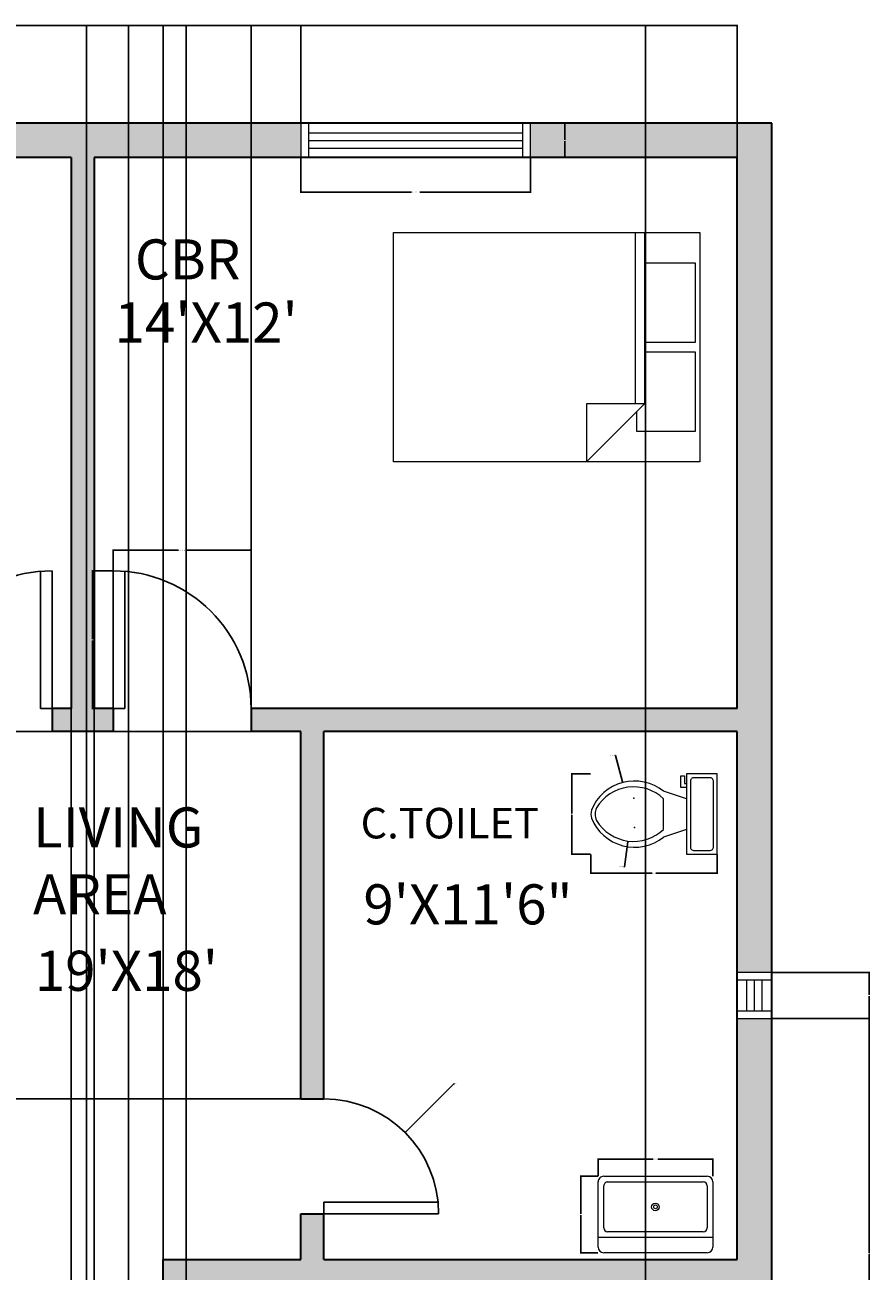
# Model space of a CAD drawing. Units: inches. Extents: x -82 to 330, y 553 to 1115.
# Tile 4 of 4: x 109 to 330, y 789 to 1115. Entities that reach past the tile are written whole.
import ezdxf

# ---------------------------------------------------------------- set-up
doc = ezdxf.new("R2010")
doc.units = ezdxf.units.IN
for name, color, linetype, lineweight in [('A-ANNO-DIMS', 2, 'Continuous', 18), ('A-AREA-IDEN', 7, 'Continuous', 25), ('A-DOOR', 3, 'Continuous', 25), ('A-FLOR-FIXT', 8, 'Continuous', 18), ('A-FURN', 8, 'Continuous', 18), ('A-GLAZ', 4, 'Continuous', 18), ('A-WALL', 7, 'Continuous', 35)]:
    doc.layers.add(name, color=color, linetype=linetype, lineweight=lineweight)
doc.layers.add('A-WALL-PATT', color=18, linetype='Continuous', lineweight=13, true_color=0x000000)
doc.styles.get("Standard").update_dxf_attribs({"font": 'arial.ttf'})
doc.dimstyles.get("Standard").update_dxf_attribs({"dimtxt": 0.18, "dimasz": 0.18, "dimexe": 0.18, "dimexo": 0.0625, "dimgap": 0.09, "dimtad": 0, "dimtih": 1, "dimtoh": 1, "dimdec": 4, "dimzin": 0, "dimdsep": 46, "dimtxsty": 'Standard', "dimcen": 0.09, "dimadec": 0, "dimazin": 0, "dimtfac": 1, "dimtdec": 4, "dimtofl": 0, "dimtmove": 0, "dimatfit": 3, "dimfxl": 1, "dimtolj": 1, "dimtzin": 0, "dimarcsym": 0})

# ---------------------------------------------------------------- blocks, each defined once
blk = doc.blocks.new('Sink-single - 30 in top')
blk.add_line((-15, -3.999996), (15, -3.999996))
for points in [[(-13.5, 0), (13.5, 0)], [(-15, -18.499996), (-15, -1.5)], [(15, -1.5), (15, -18.499996)], [(-13.5, -17.499996), (-13.5, -6.499996)], [(-12.5, -5.499996), (12.5, -5.499996)], [(13.5, -6.499996), (13.5, -17.499996)], [(12.5, -18.499996), (-12.5, -18.499996)], [(13.5, -19.999996), (-13.5, -19.999996)]]:
    blk.add_lwpolyline(points)
for radius in [1, 0.5]:
    blk.add_circle((0, -11.999996), radius)
for centre, radius, start, end in [((-13.5, -1.5), 1.5, 90, 180), ((13.5, -1.5), 1.5, 0, 90), ((-12.5, -6.499996), 1, 90, 180), ((12.5, -6.499996), 1, 0, 90), ((-13.5, -18.499996), 1.5, 180, 270), ((-12.5, -17.499996), 1, 180, 270), ((12.5, -17.499996), 1, 270, 0), ((13.5, -18.499996), 1.5, 270, 0)]:
    blk.add_arc(centre, radius, start, end)
blk = doc.blocks.new('Bed - Queen')
for p, q in [((0, -80.00003), (0, 0)), ((0, 0), (59.99999, 0)), ((59.99999, 0), (59.99999, -80.00003)), ((7.99999, -1.2), (28.79998, -1.2)), ((7.99999, -14.4), (7.99999, -1.2)), ((28.79998, -1.2), (28.79998, -14.4)), ((31.19999, -1.2), (51.99999, -1.2)), ((31.19999, -14.4), (31.19999, -1.2)), ((51.99999, -1.2), (51.99999, -16.4)), ((0, -14.4), (44.8, -14.4)), ((59.99999, -29.6), (44.8, -14.4)), ((44.8, -14.4), (44.8, -29.6)), ((44.8, -16.8), (0, -16.8)), ((51.99999, -16.4), (46.79936, -16.4)), ((44.8, -29.6), (59.99999, -29.6)), ((59.99999, -80.00003), (0, -80.00003))]:
    blk.add_line(p, q)
blk = doc.blocks.new('Toilet - top')
for p, q in [((9.5, -6), (9.5, -2)), ((-10, -8.5), (-8, -8.5)), ((-10, -9.5), (-10, -8.5)), ((-7, -9.5), (-10, -9.5)), ((-8, -8.5), (-8, -8)), ((-7, -8), (-7, -9.5)), ((-4, -8), (-6, -14)), ((4, -8), (6, -14)), ((4, -14), (-4, -14))]:
    blk.add_line(p, q)
blk.add_lwpolyline([(10.5, -8), (10.5, 0), (-10.5, 0), (-10.5, -8)], close=True)
for points in [[(-9.5, -2), (-9.5, -6)], [(8.5, -1), (-8.5, -1)], [(-8.5, -7), (8.5, -7)]]:
    blk.add_lwpolyline(points)
for centre, radius, start, end in [((-8.62, -1.88), 0.884, 81.8699, 188.1301), ((8.62, -1.88), 0.884, 351.8699, 98.1301), ((-8.62, -6.12), 0.884, 171.8699, 278.1301), ((8.62, -6.12), 0.884, 261.8699, 8.1301), ((3.52, -21.58), 12.17, 141.4691, 247.9714), ((4.2, -21.82), 11.33, 136.3677, 238.9468), ((-3.52, -21.58), 12.17, 292.0284, 38.5307), ((-4.2, -21.82), 11.33, 301.053, 43.6321), ((0, -27.88), 4, 245.7318, 294.2682), ((0, -29), 4, 254.8605, 285.1395)]:
    blk.add_arc(centre, radius, start, end)
blk = doc.blocks.new('WIN-60IN')
for p, q in [((60, 9), (0, 9)), ((0, 9), (0, 0)), ((2, 9), (2, 0)), ((58, 0), (58, 9)), ((60, 0), (60, 9)), ((2, 6.5), (58, 6.5)), ((2, 4.5), (58, 4.5)), ((0, 0), (60, 0)), ((2, 2.5), (58, 2.5))]:
    blk.add_line(p, q)
blk = doc.blocks.new('DOOR-SWING-36IN')
for p, q in [((0, 36), (0, 0)), ((3, 36), (3, 0)), ((0, 0), (3, 0))]:
    blk.add_line(p, q)
blk.add_arc((0, 0), 36, 0, 90)
blk = doc.blocks.new('*D11')
at = {"layer": 'A-ANNO-DIMS', "color": 0, "lineweight": -2, "transparency": 16777216}
for p, q in [((180.99, 1080.05), (180.99, 1070.93)), ((240.99, 1080.05), (240.99, 1070.93)), ((181.17, 1071.11), (209.87, 1071.11)), ((240.81, 1071.11), (212.11, 1071.11))]:
    blk.add_line(p, q, dxfattribs=at)
at = {"layer": 'A-ANNO-DIMS', "color": 0, "transparency": 16777216}
for points in [[(181.17, 1071.14), (181.17, 1071.08), (180.99, 1071.11)], [(240.81, 1071.14), (240.81, 1071.08), (240.99, 1071.11)]]:
    blk.add_solid(points, dxfattribs=at)
at = {"layer": 'Defpoints', "color": 0, "transparency": 16777216}
for p in [(180.99, 1080.11), (240.99, 1080.11), (240.99, 1071.11)]:
    blk.add_point(p, dxfattribs=at)
at = {"layer": 'A-ANNO-DIMS', "color": 0, "transparency": 16777216, "insert": (210.99, 1071.11), "char_height": 0.18, "attachment_point": 5}
blk.add_mtext('\\A1;WINDOW 60 TYP.', dxfattribs=at)
blk = doc.blocks.new('*D12')
at = {"layer": 'A-ANNO-DIMS', "color": 0, "lineweight": -2, "transparency": 16777216}
for p, q in [((241.05, 1089.11), (250.17, 1089.11)), ((249.99, 1088.93), (249.99, 1084.79)), ((249.99, 1080.29), (249.99, 1084.43)), ((241.05, 1080.11), (250.17, 1080.11))]:
    blk.add_line(p, q, dxfattribs=at)
at = {"layer": 'A-ANNO-DIMS', "color": 0, "transparency": 16777216}
for points in [[(249.96, 1088.93), (250.02, 1088.93), (249.99, 1089.11)], [(249.96, 1080.29), (250.02, 1080.29), (249.99, 1080.11)]]:
    blk.add_solid(points, dxfattribs=at)
at = {"layer": 'Defpoints', "color": 0, "transparency": 16777216}
for p in [(240.99, 1089.11), (249.99, 1089.11), (240.99, 1080.11)]:
    blk.add_point(p, dxfattribs=at)
at = {"layer": 'A-ANNO-DIMS', "color": 0, "transparency": 16777216, "insert": (249.99, 1084.61), "char_height": 0.18, "attachment_point": 5}
blk.add_mtext('\\A1;9 TYP.', dxfattribs=at)
blk = doc.blocks.new('*D13')
at = {"layer": 'A-ANNO-DIMS', "color": 0, "lineweight": -2, "transparency": 16777216}
for p, q in [((131.99, 972.17), (131.99, 977.69)), ((132.17, 977.51), (149.05, 977.51)), ((167.81, 977.51), (150.92, 977.51)), ((167.99, 972.17), (167.99, 977.69))]:
    blk.add_line(p, q, dxfattribs=at)
at = {"layer": 'A-ANNO-DIMS', "color": 0, "transparency": 16777216}
for points in [[(132.17, 977.54), (132.17, 977.48), (131.99, 977.51)], [(167.81, 977.54), (167.81, 977.48), (167.99, 977.51)]]:
    blk.add_solid(points, dxfattribs=at)
at = {"layer": 'Defpoints', "color": 0, "transparency": 16777216}
for p in [(167.99, 977.51), (131.99, 972.11), (167.99, 972.11)]:
    blk.add_point(p, dxfattribs=at)
at = {"layer": 'A-ANNO-DIMS', "color": 0, "transparency": 16777216, "insert": (149.99, 977.51), "char_height": 0.18, "attachment_point": 5}
blk.add_mtext('\\A1;DOOR 36 TYP.', dxfattribs=at)
blk = doc.blocks.new('*D14')
at = {"layer": 'A-ANNO-DIMS', "color": 0, "lineweight": -2, "transparency": 16777216}
for p, q in [((131.93, 972.11), (126.41, 972.11)), ((126.59, 971.93), (126.59, 954.29)), ((126.59, 936.29), (126.59, 953.93)), ((131.93, 936.11), (126.41, 936.11))]:
    blk.add_line(p, q, dxfattribs=at)
at = {"layer": 'A-ANNO-DIMS', "color": 0, "transparency": 16777216}
for points in [[(126.56, 971.93), (126.62, 971.93), (126.59, 972.11)], [(126.56, 936.29), (126.62, 936.29), (126.59, 936.11)]]:
    blk.add_solid(points, dxfattribs=at)
at = {"layer": 'Defpoints', "color": 0, "transparency": 16777216}
for p in [(126.59, 972.11), (131.99, 972.11), (131.99, 936.11)]:
    blk.add_point(p, dxfattribs=at)
at = {"layer": 'A-ANNO-DIMS', "color": 0, "transparency": 16777216, "insert": (126.59, 954.11), "char_height": 0.18, "attachment_point": 5}
blk.add_mtext('\\A1;36 TYP.', dxfattribs=at)
blk = doc.blocks.new('*D23')
at = {"layer": 'A-ANNO-DIMS', "color": 0, "lineweight": -2, "transparency": 16777216}
for p, q in [((258.63, 813.95), (258.63, 818.57)), ((258.81, 818.39), (273, 818.39)), ((288.45, 818.39), (274.26, 818.39)), ((288.63, 813.95), (288.63, 818.57))]:
    blk.add_line(p, q, dxfattribs=at)
at = {"layer": 'A-ANNO-DIMS', "color": 0, "transparency": 16777216}
for points in [[(258.81, 818.42), (258.81, 818.36), (258.63, 818.39)], [(288.45, 818.42), (288.45, 818.36), (288.63, 818.39)]]:
    blk.add_solid(points, dxfattribs=at)
at = {"layer": 'Defpoints', "color": 0, "transparency": 16777216}
for p in [(258.63, 818.39), (258.63, 813.89), (288.63, 813.89)]:
    blk.add_point(p, dxfattribs=at)
at = {"layer": 'A-ANNO-DIMS', "color": 0, "transparency": 16777216, "insert": (273.63, 818.39), "char_height": 0.18, "attachment_point": 5}
blk.add_mtext('\\A1;BASIN 30', dxfattribs=at)
blk = doc.blocks.new('*D24')
at = {"layer": 'A-ANNO-DIMS', "color": 0, "lineweight": -2, "transparency": 16777216}
for p, q in [((258.57, 813.89), (253.95, 813.89)), ((254.13, 813.71), (254.13, 804.07)), ((254.13, 794.07), (254.13, 803.71)), ((258.57, 793.89), (253.95, 793.89))]:
    blk.add_line(p, q, dxfattribs=at)
at = {"layer": 'A-ANNO-DIMS', "color": 0, "transparency": 16777216}
for points in [[(254.1, 813.71), (254.16, 813.71), (254.13, 813.89)], [(254.1, 794.07), (254.16, 794.07), (254.13, 793.89)]]:
    blk.add_solid(points, dxfattribs=at)
at = {"layer": 'Defpoints', "color": 0, "transparency": 16777216}
for p in [(258.63, 813.89), (254.13, 793.89), (258.63, 793.89)]:
    blk.add_point(p, dxfattribs=at)
at = {"layer": 'A-ANNO-DIMS', "color": 0, "transparency": 16777216, "insert": (254.13, 803.89), "char_height": 0.18, "attachment_point": 5}
blk.add_mtext('\\A1;20', dxfattribs=at)
blk = doc.blocks.new('*D29')
at = {"layer": 'A-ANNO-DIMS', "color": 0, "lineweight": -2, "transparency": 16777216}
for p, q in [((256.71, 897.97), (256.71, 892.9)), ((289.76, 897.97), (289.76, 892.9)), ((256.89, 893.08), (272.77, 893.08)), ((289.58, 893.08), (273.7, 893.08))]:
    blk.add_line(p, q, dxfattribs=at)
at = {"layer": 'A-ANNO-DIMS', "color": 0, "transparency": 16777216}
for points in [[(256.89, 893.11), (256.89, 893.05), (256.71, 893.08)], [(289.58, 893.11), (289.58, 893.05), (289.76, 893.08)]]:
    blk.add_solid(points, dxfattribs=at)
at = {"layer": 'Defpoints', "color": 0, "transparency": 16777216}
for p in [(256.71, 898.03), (289.76, 898.03), (289.76, 893.08)]:
    blk.add_point(p, dxfattribs=at)
at = {"layer": 'A-ANNO-DIMS', "color": 0, "transparency": 16777216, "insert": (273.23, 893.08), "char_height": 0.18, "attachment_point": 5}
blk.add_mtext('\\A1;WC 33', dxfattribs=at)
blk = doc.blocks.new('*D30')
at = {"layer": 'A-ANNO-DIMS', "color": 0, "lineweight": -2, "transparency": 16777216}
for p, q in [((256.65, 919.03), (251.57, 919.03)), ((251.75, 918.85), (251.75, 908.72)), ((251.75, 898.21), (251.75, 908.35)), ((256.65, 898.03), (251.57, 898.03))]:
    blk.add_line(p, q, dxfattribs=at)
at = {"layer": 'A-ANNO-DIMS', "color": 0, "transparency": 16777216}
for points in [[(251.72, 918.85), (251.78, 918.85), (251.75, 919.03)], [(251.72, 898.21), (251.78, 898.21), (251.75, 898.03)]]:
    blk.add_solid(points, dxfattribs=at)
at = {"layer": 'Defpoints', "color": 0, "transparency": 16777216}
for p in [(256.71, 919.03), (251.75, 898.03), (256.71, 898.03)]:
    blk.add_point(p, dxfattribs=at)
at = {"layer": 'A-ANNO-DIMS', "color": 0, "transparency": 16777216, "insert": (251.75, 908.53), "char_height": 0.18, "attachment_point": 5}
blk.add_mtext('\\A1;21', dxfattribs=at)
blk = doc.blocks.new('*D34')
at = {"layer": 'A-ANNO-DIMS', "color": 0, "lineweight": -2, "transparency": 16777216}
for p, q in [((66.99, 1089.17), (66.99, 1114.79)), ((67.17, 1114.61), (123.71, 1114.61)), ((180.81, 1114.61), (124.27, 1114.61)), ((180.99, 1089.17), (180.99, 1114.79))]:
    blk.add_line(p, q, dxfattribs=at)
at = {"layer": 'A-ANNO-DIMS', "color": 0, "transparency": 16777216}
for points in [[(67.17, 1114.64), (67.17, 1114.58), (66.99, 1114.61)], [(180.81, 1114.64), (180.81, 1114.58), (180.99, 1114.61)]]:
    blk.add_solid(points, dxfattribs=at)
at = {"layer": 'Defpoints', "color": 0, "transparency": 16777216}
for p in [(180.99, 1114.61), (66.99, 1089.11), (180.99, 1089.11)]:
    blk.add_point(p, dxfattribs=at)
at = {"layer": 'A-ANNO-DIMS', "color": 0, "transparency": 16777216, "insert": (123.99, 1114.61), "char_height": 0.18, "attachment_point": 5}
blk.add_mtext('\\A1;114', dxfattribs=at)
blk = doc.blocks.new('*D35')
at = {"layer": 'A-ANNO-DIMS', "color": 0, "lineweight": -2, "transparency": 16777216}
for p, q in [((84.99, 627.17), (84.99, 1114.79)), ((85.17, 1114.61), (110.29, 1114.61)), ((135.81, 1114.61), (110.69, 1114.61)), ((135.99, 618.17), (135.99, 1114.79))]:
    blk.add_line(p, q, dxfattribs=at)
at = {"layer": 'A-ANNO-DIMS', "color": 0, "transparency": 16777216}
for points in [[(85.17, 1114.64), (85.17, 1114.58), (84.99, 1114.61)], [(135.81, 1114.64), (135.81, 1114.58), (135.99, 1114.61)]]:
    blk.add_solid(points, dxfattribs=at)
at = {"layer": 'Defpoints', "color": 0, "transparency": 16777216}
for p in [(135.99, 1114.61), (84.99, 627.11), (135.99, 618.11)]:
    blk.add_point(p, dxfattribs=at)
at = {"layer": 'A-ANNO-DIMS', "color": 0, "transparency": 16777216, "insert": (110.49, 1114.61), "char_height": 0.18, "attachment_point": 5}
blk.add_mtext('\\A1;51', dxfattribs=at)
blk = doc.blocks.new('*D39')
at = {"layer": 'A-ANNO-DIMS', "color": 0, "lineweight": -2, "transparency": 16777216}
for p, q in [((304.05, 855.11), (329.67, 855.11)), ((329.49, 854.93), (329.49, 793.79)), ((329.49, 732.29), (329.49, 793.43)), ((304.05, 732.11), (329.67, 732.11))]:
    blk.add_line(p, q, dxfattribs=at)
at = {"layer": 'A-ANNO-DIMS', "color": 0, "transparency": 16777216}
for points in [[(329.46, 854.93), (329.52, 854.93), (329.49, 855.11)], [(329.46, 732.29), (329.52, 732.29), (329.49, 732.11)]]:
    blk.add_solid(points, dxfattribs=at)
at = {"layer": 'Defpoints', "color": 0, "transparency": 16777216}
for p in [(303.99, 855.11), (329.49, 855.11), (303.99, 732.11)]:
    blk.add_point(p, dxfattribs=at)
at = {"layer": 'A-ANNO-DIMS', "color": 0, "transparency": 16777216, "insert": (329.49, 793.61), "char_height": 0.18, "attachment_point": 5}
blk.add_mtext('\\A1;123', dxfattribs=at)
blk = doc.blocks.new('*D40')
at = {"layer": 'A-ANNO-DIMS', "color": 0, "lineweight": -2, "transparency": 16777216}
for p, q in [((304.05, 867.11), (329.67, 867.11)), ((329.49, 866.93), (329.49, 861.29)), ((329.49, 855.29), (329.49, 860.93)), ((304.05, 855.11), (329.67, 855.11))]:
    blk.add_line(p, q, dxfattribs=at)
at = {"layer": 'A-ANNO-DIMS', "color": 0, "transparency": 16777216}
for points in [[(329.46, 866.93), (329.52, 866.93), (329.49, 867.11)], [(329.46, 855.29), (329.52, 855.29), (329.49, 855.11)]]:
    blk.add_solid(points, dxfattribs=at)
at = {"layer": 'Defpoints', "color": 0, "transparency": 16777216}
for p in [(303.99, 867.11), (329.49, 867.11), (303.99, 855.11)]:
    blk.add_point(p, dxfattribs=at)
at = {"layer": 'A-ANNO-DIMS', "color": 0, "transparency": 16777216, "insert": (329.49, 861.11), "char_height": 0.18, "attachment_point": 5}
blk.add_mtext('\\A1;12', dxfattribs=at)
blk = doc.blocks.new('*D41')
at = {"layer": 'A-ANNO-DIMS', "color": 0, "lineweight": -2, "transparency": 16777216}
for p, q in [((124.99, 714.17), (124.99, 1114.79)), ((125.17, 1114.61), (134.77, 1114.61)), ((144.81, 1114.61), (135.21, 1114.61)), ((144.99, 714.17), (144.99, 1114.79))]:
    blk.add_line(p, q, dxfattribs=at)
at = {"layer": 'A-ANNO-DIMS', "color": 0, "transparency": 16777216}
for points in [[(125.17, 1114.64), (125.17, 1114.58), (124.99, 1114.61)], [(144.81, 1114.64), (144.81, 1114.58), (144.99, 1114.61)]]:
    blk.add_solid(points, dxfattribs=at)
at = {"layer": 'Defpoints', "color": 0, "transparency": 16777216}
for p in [(144.99, 1114.61), (124.99, 714.11), (144.99, 714.11)]:
    blk.add_point(p, dxfattribs=at)
at = {"layer": 'A-ANNO-DIMS', "color": 0, "transparency": 16777216, "insert": (134.99, 1114.61), "char_height": 0.18, "attachment_point": 5}
blk.add_mtext('\\A1;20', dxfattribs=at)
blk = doc.blocks.new('*D43')
at = {"layer": 'A-ANNO-DIMS', "color": 0, "lineweight": -2, "transparency": 16777216}
for p, q in [((120.99, 1080.05), (120.99, 553.43)), ((126.99, 1080.05), (126.99, 553.43)), ((121.17, 553.61), (123.84, 553.61)), ((126.81, 553.61), (124.14, 553.61))]:
    blk.add_line(p, q, dxfattribs=at)
at = {"layer": 'A-ANNO-DIMS', "color": 0, "transparency": 16777216}
for points in [[(121.17, 553.64), (121.17, 553.58), (120.99, 553.61)], [(126.81, 553.64), (126.81, 553.58), (126.99, 553.61)]]:
    blk.add_solid(points, dxfattribs=at)
at = {"layer": 'Defpoints', "color": 0, "transparency": 16777216}
for p in [(120.99, 1080.11), (126.99, 1080.11), (126.99, 553.61)]:
    blk.add_point(p, dxfattribs=at)
at = {"layer": 'A-ANNO-DIMS', "color": 0, "transparency": 16777216, "insert": (123.99, 553.61), "char_height": 0.18, "attachment_point": 5}
blk.add_mtext('\\A1;6', dxfattribs=at)
blk = doc.blocks.new('*D45')
at = {"layer": 'A-ANNO-DIMS', "color": 0, "lineweight": -2, "transparency": 16777216}
for p, q in [((180.93, 930.11), (-81.69, 930.11)), ((-81.51, 929.93), (-81.51, 882.29)), ((-81.51, 834.29), (-81.51, 881.93)), ((180.93, 834.11), (-81.69, 834.11))]:
    blk.add_line(p, q, dxfattribs=at)
at = {"layer": 'A-ANNO-DIMS', "color": 0, "transparency": 16777216}
for points in [[(-81.54, 929.93), (-81.48, 929.93), (-81.51, 930.11)], [(-81.54, 834.29), (-81.48, 834.29), (-81.51, 834.11)]]:
    blk.add_solid(points, dxfattribs=at)
at = {"layer": 'Defpoints', "color": 0, "transparency": 16777216}
for p in [(180.99, 930.11), (-81.51, 834.11), (180.99, 834.11)]:
    blk.add_point(p, dxfattribs=at)
at = {"layer": 'A-ANNO-DIMS', "color": 0, "transparency": 16777216, "insert": (-81.51, 882.11), "char_height": 0.18, "attachment_point": 5}
blk.add_mtext('\\A1;96', dxfattribs=at)
blk = doc.blocks.new('*D47')
at = {"layer": 'A-ANNO-DIMS', "color": 0, "lineweight": -2, "transparency": 16777216}
for p, q in [((167.99, 936.17), (167.99, 1114.79)), ((168.17, 1114.61), (231.21, 1114.61)), ((294.81, 1114.61), (231.77, 1114.61)), ((294.99, 936.17), (294.99, 1114.79))]:
    blk.add_line(p, q, dxfattribs=at)
at = {"layer": 'A-ANNO-DIMS', "color": 0, "transparency": 16777216}
for points in [[(168.17, 1114.64), (168.17, 1114.58), (167.99, 1114.61)], [(294.81, 1114.64), (294.81, 1114.58), (294.99, 1114.61)]]:
    blk.add_solid(points, dxfattribs=at)
at = {"layer": 'Defpoints', "color": 0, "transparency": 16777216}
for p in [(294.99, 1114.61), (167.99, 936.11), (294.99, 936.11)]:
    blk.add_point(p, dxfattribs=at)
at = {"layer": 'A-ANNO-DIMS', "color": 0, "transparency": 16777216, "insert": (231.49, 1114.61), "char_height": 0.18, "attachment_point": 5}
blk.add_mtext('\\A1;127', dxfattribs=at)
blk = doc.blocks.new('*D48')
at = {"layer": 'A-ANNO-DIMS', "color": 0, "lineweight": -2, "transparency": 16777216}
for p, q in [((-50.01, 609.17), (-50.01, 1114.79)), ((-49.83, 1114.61), (42.71, 1114.61)), ((135.81, 1114.61), (43.27, 1114.61)), ((135.99, 618.17), (135.99, 1114.79))]:
    blk.add_line(p, q, dxfattribs=at)
at = {"layer": 'A-ANNO-DIMS', "color": 0, "transparency": 16777216}
for points in [[(-49.83, 1114.64), (-49.83, 1114.58), (-50.01, 1114.61)], [(135.81, 1114.64), (135.81, 1114.58), (135.99, 1114.61)]]:
    blk.add_solid(points, dxfattribs=at)
at = {"layer": 'Defpoints', "color": 0, "transparency": 16777216}
for p in [(135.99, 1114.61), (135.99, 618.11), (-50.01, 609.11)]:
    blk.add_point(p, dxfattribs=at)
at = {"layer": 'A-ANNO-DIMS', "color": 0, "transparency": 16777216, "insert": (42.99, 1114.61), "char_height": 0.18, "attachment_point": 5}
blk.add_mtext('\\A1;186', dxfattribs=at)
blk = doc.blocks.new('*D49')
at = {"layer": 'A-ANNO-DIMS', "color": 0, "lineweight": -2, "transparency": 16777216}
for p, q in [((150.99, 642.17), (150.99, 1114.79)), ((151.17, 1114.61), (210.71, 1114.61)), ((270.81, 1114.61), (211.27, 1114.61)), ((270.99, 642.17), (270.99, 1114.79))]:
    blk.add_line(p, q, dxfattribs=at)
at = {"layer": 'A-ANNO-DIMS', "color": 0, "transparency": 16777216}
for points in [[(151.17, 1114.64), (151.17, 1114.58), (150.99, 1114.61)], [(270.81, 1114.64), (270.81, 1114.58), (270.99, 1114.61)]]:
    blk.add_solid(points, dxfattribs=at)
at = {"layer": 'Defpoints', "color": 0, "transparency": 16777216}
for p in [(270.99, 1114.61), (150.99, 642.11), (270.99, 642.11)]:
    blk.add_point(p, dxfattribs=at)
at = {"layer": 'A-ANNO-DIMS', "color": 0, "transparency": 16777216, "insert": (210.99, 1114.61), "char_height": 0.18, "attachment_point": 5}
blk.add_mtext('\\A1;120', dxfattribs=at)
blk = doc.blocks.new('*D51')
at = {"layer": 'A-ANNO-DIMS', "color": 0, "lineweight": -2, "transparency": 16777216}
for p, q in [((220.93, 838.05), (208.33, 825.45)), ((221.11, 838.05), (220.93, 838.05)), ((186.9, 804.11), (187.08, 804.11)), ((186.99, 804.02), (186.99, 804.2))]:
    blk.add_line(p, q, dxfattribs=at)
at = {"layer": 'A-ANNO-DIMS', "color": 0, "transparency": 16777216}
blk.add_solid([(208.31, 825.47), (208.35, 825.43), (208.2, 825.32)], dxfattribs=at)
at = {"layer": 'Defpoints', "color": 0, "transparency": 16777216}
for p in [(208.2, 825.32), (186.99, 804.11)]:
    blk.add_point(p, dxfattribs=at)
at = {"layer": 'A-ANNO-DIMS', "color": 0, "transparency": 16777216, "insert": (221.41, 838.05), "char_height": 0.18, "attachment_point": 5}
blk.add_mtext('\\A1;R30', dxfattribs=at)
blk = doc.blocks.new('*D52')
at = {"layer": 'A-ANNO-DIMS', "color": 0, "lineweight": -2, "transparency": 16777216}
for p, q in [((263.05, 923.85), (263.23, 923.85)), ((263.23, 923.85), (265.04, 916.96)), ((268.09, 905.02), (268.27, 905.02)), ((268.18, 904.93), (268.18, 905.11))]:
    blk.add_line(p, q, dxfattribs=at)
at = {"layer": 'A-ANNO-DIMS', "color": 0, "transparency": 16777216}
blk.add_solid([(265.07, 916.97), (265.01, 916.95), (265.08, 916.78)], dxfattribs=at)
at = {"layer": 'Defpoints', "color": 0, "transparency": 16777216}
for p in [(265.08, 916.78), (268.18, 905.02)]:
    blk.add_point(p, dxfattribs=at)
at = {"layer": 'A-ANNO-DIMS', "color": 0, "transparency": 16777216, "insert": (262.37, 923.85), "char_height": 0.18, "attachment_point": 5}
blk.add_mtext('\\A1;2X R12.17', dxfattribs=at)
blk = doc.blocks.new('*D53')
at = {"layer": 'A-ANNO-DIMS', "color": 0, "lineweight": -2, "transparency": 16777216}
for p, q in [((267.85, 912.73), (268.03, 912.73)), ((267.94, 912.64), (267.94, 912.82)), ((265.52, 894.77), (266.41, 901.33)), ((265.34, 894.77), (265.52, 894.77))]:
    blk.add_line(p, q, dxfattribs=at)
at = {"layer": 'A-ANNO-DIMS', "color": 0, "transparency": 16777216}
blk.add_solid([(266.38, 901.33), (266.43, 901.32), (266.43, 901.51)], dxfattribs=at)
at = {"layer": 'Defpoints', "color": 0, "transparency": 16777216}
for p in [(267.94, 912.73), (266.43, 901.51)]:
    blk.add_point(p, dxfattribs=at)
at = {"layer": 'A-ANNO-DIMS', "color": 0, "transparency": 16777216, "insert": (264.67, 894.77), "char_height": 0.18, "attachment_point": 5}
blk.add_mtext('\\A1;2X R11.33', dxfattribs=at)

msp = doc.modelspace()

# ---------------------------------------------------------------- hatches: boundary and pattern name
at = {"layer": 'A-WALL-PATT'}
h = msp.add_hatch(color=256, dxfattribs=at)
h.dxf.hatch_style = 1
h.paths.add_polyline_path([(6.988, 1089.11), (-56.012, 1089.11), (-56.012, 705.11), (-47.012, 705.11), (-15.012, 705.11), (-15.012, 714.11), (-47.012, 714.11), (-47.012, 930.11), (79.988, 930.11), (79.988, 936.11), (-47.012, 936.11), (-47.012, 1080.11), (6.988, 1080.11)])
h.paths.add_polyline_path([(180.988, 1089.11), (66.988, 1089.11), (66.988, 1080.11), (120.988, 1080.11), (120.988, 936.11), (115.988, 936.11), (115.988, 930.11), (131.988, 930.11), (131.988, 936.11), (126.988, 936.11), (126.988, 1080.11), (180.988, 1080.11)])
h.paths.add_polyline_path([(303.988, 1089.11), (240.988, 1089.11), (240.988, 1080.11), (294.988, 1080.11), (294.988, 936.11), (167.988, 936.11), (167.988, 930.11), (180.988, 930.11), (180.988, 834.11), (186.988, 834.11), (186.988, 930.11), (294.988, 930.11), (294.988, 867.11), (303.988, 867.11)])
h.paths.add_polyline_path([(303.988, 855.11), (294.988, 855.11), (294.988, 792.11), (186.988, 792.11), (186.988, 804.11), (180.988, 804.11), (180.988, 792.11), (144.988, 792.11), (144.988, 756.11), (150.988, 756.11), (150.988, 786.11), (294.988, 786.11), (294.988, 732.11), (303.988, 732.11)])
h.paths.add_polyline_path([(303.988, 672.11), (294.988, 672.11), (294.988, 618.11), (150.988, 618.11), (150.988, 720.11), (144.988, 720.11), (144.988, 714.11), (124.988, 714.11), (124.988, 705.11), (144.988, 705.11), (144.988, 618.11), (144.988, 609.11), (303.988, 609.11)])
h.paths.add_polyline_path([(76.988, 714.11), (44.988, 714.11), (44.988, 705.11), (76.988, 705.11)], flags=17)

# ---------------------------------------------------------------- linework, layer by layer
at = {"layer": 'A-DOOR'}
for p, q in [((216.988, 807.11), (186.988, 807.11)), ((186.988, 804.11), (186.988, 807.11)), ((216.988, 804.11), (186.988, 804.11))]:
    msp.add_line(p, q, dxfattribs=at)
msp.add_arc((186.988, 804.11), 30, 0, 90, dxfattribs=at)
at = {"layer": 'A-GLAZ'}
for p, q in [((303.988, 867.11), (294.988, 867.11)), ((294.988, 867.11), (294.988, 855.11)), ((303.988, 855.11), (303.988, 867.11)), ((303.988, 865.11), (294.988, 865.11)), ((297.488, 857.11), (297.488, 865.11)), ((299.488, 857.11), (299.488, 865.11)), ((301.488, 857.11), (301.488, 865.11)), ((294.988, 857.11), (303.988, 857.11)), ((294.988, 855.11), (303.988, 855.11))]:
    msp.add_line(p, q, dxfattribs=at)
at = {"layer": 'A-WALL'}
for p, q in [((303.988, 1089.11), (-56.012, 1089.11)), ((303.988, 609.11), (303.988, 1089.11)), ((120.988, 1080.11), (-47.012, 1080.11)), ((120.988, 1080.11), (120.988, 936.11)), ((294.988, 1080.11), (126.988, 1080.11)), ((126.988, 1080.11), (126.988, 936.11)), ((294.988, 936.11), (294.988, 1080.11)), ((115.988, 936.11), (115.988, 930.11)), ((120.988, 936.11), (115.988, 936.11)), ((131.988, 936.11), (126.988, 936.11)), ((131.988, 936.11), (131.988, 930.11)), ((294.988, 936.11), (167.988, 936.11)), ((167.988, 936.11), (167.988, 930.11)), ((131.988, 930.11), (115.988, 930.11)), ((180.988, 930.11), (167.988, 930.11)), ((180.988, 834.11), (180.988, 930.11)), ((294.988, 930.11), (186.988, 930.11)), ((186.988, 834.11), (186.988, 930.11)), ((294.988, 792.11), (294.988, 930.11)), ((180.988, 834.11), (186.988, 834.11)), ((180.988, 792.11), (180.988, 804.11)), ((180.988, 804.11), (186.988, 804.11)), ((186.988, 792.11), (186.988, 804.11)), ((144.988, 792.11), (180.988, 792.11)), ((144.988, 756.11), (144.988, 792.11)), ((186.988, 792.11), (294.988, 792.11))]:
    msp.add_line(p, q, dxfattribs=at)

# ---------------------------------------------------------------- block references
at = {"layer": 'A-DOOR', "extrusion": (0, 0, -1), "zscale": -1}
msp.add_blockref('DOOR-SWING-36IN', (-115.989, 936.11), dxfattribs=at)
at = {"layer": 'A-DOOR'}
msp.add_blockref('DOOR-SWING-36IN', (131.988, 936.11), dxfattribs=at)
at = {"layer": 'A-FLOR-FIXT'}
for name, p, rotation in [('Toilet - top', (289.756, 908.535), 270), ('Sink-single - 30 in top', (273.628, 793.892), 180)]:
    msp.add_blockref(name, p, dxfattribs=dict(at, rotation=rotation))
at = {"layer": 'A-FURN', "rotation": 270}
msp.add_blockref('Bed - Queen', (285.187, 1060.575), dxfattribs=at)
at = {"layer": 'A-GLAZ'}
msp.add_blockref('WIN-60IN', (180.988, 1080.11), dxfattribs=at)

# ---------------------------------------------------------------- texts
at = {"layer": 'A-AREA-IDEN', "attachment_point": 1}
for s, width, gutter_width, insert, char_height in [('CBR', 470.55254, 52.378, (137.648, 1058.743), 10.4756), ("14'X12'", 470.55254, 52.378, (132.313, 1042.248), 10.4756), ('LIVING\\PAREA', 470.55254, 52.378, (111.028, 910.29), 10.4756), ('C.TOILET', 358.39781, 39.894, (196.6, 910.161), 7.9787), ('9\'X11\'6"', 470.55254, 52.378, (197.322, 890.19), 10.4756), ("19'X18'", 470.55254, 52.378, (111.491, 872.819), 10.4756)]:
    msp.add_mtext_dynamic_manual_height_columns(s, width=width, gutter_width=gutter_width, heights=[0], dxfattribs=dict(at, insert=insert, char_height=char_height))

# ---------------------------------------------------------------- dimensions: what is measured, and where the dimension line sits
at = {"layer": 'A-ANNO-DIMS'}
for base, p1, p2, picture, middle in [((135.988, 1114.611), (-50.012, 609.11), (135.988, 618.11), '*D48', (42.988, 1114.611)), ((180.988, 1114.611), (66.988, 1089.11), (180.988, 1089.11), '*D34', (123.988, 1114.611)), ((135.988, 1114.611), (84.988, 627.11), (135.988, 618.11), '*D35', (110.488, 1114.611)), ((144.988, 1114.611), (124.988, 714.11), (144.988, 714.11), '*D41', (134.988, 1114.611)), ((270.988, 1114.611), (150.988, 642.11), (270.988, 642.11), '*D49', (210.988, 1114.611)), ((294.988, 1114.611), (167.988, 936.11), (294.988, 936.11), '*D47', (231.488, 1114.611)), ((126.988, 553.609), (120.988, 1080.11), (126.988, 1080.11), '*D43', (123.988, 553.609))]:
    dim = msp.add_linear_dim(base=base, p1=p1, p2=p2, dimstyle='Standard', override={"dimdec": 0, "dimlfac": 1, "dimrnd": 0, "dimzin": 0, "dimdsep": 46, "dimlunit": 2}, dxfattribs=at)
    dim.commit()
    dim.dimension.update_dxf_attribs({"geometry": picture, "text_midpoint": middle})
for base, p1, p2, angle, text, picture, middle in [((249.988, 1089.11), (240.988, 1080.11), (240.988, 1089.11), 90, '<> TYP.', '*D12', (249.988, 1084.61)), ((126.588, 972.11), (131.988, 936.11), (131.988, 972.11), 90, '<> TYP.', '*D14', (126.588, 954.11)), ((258.628, 818.392), (288.628, 813.892), (258.628, 813.892), 180, 'BASIN <>', '*D23', (273.628, 818.392))]:
    dim = msp.add_linear_dim(base=base, p1=p1, p2=p2, angle=angle, text=text, dimstyle='Standard', override={"dimdec": 0, "dimlfac": 1, "dimrnd": 0, "dimzin": 0, "dimdsep": 46, "dimlunit": 2}, dxfattribs=at)
    dim.commit()
    dim.dimension.update_dxf_attribs({"geometry": picture, "text_midpoint": middle})
for base, p1, p2, text, picture, middle in [((240.988, 1071.11), (180.988, 1080.11), (240.988, 1080.11), 'WINDOW <> TYP.', '*D11', (210.988, 1071.11)), ((167.988, 977.51), (131.988, 972.11), (167.988, 972.11), 'DOOR <> TYP.', '*D13', (149.988, 977.51)), ((289.756, 893.078), (256.71, 898.035), (289.756, 898.035), 'WC <>', '*D29', (273.233, 893.078))]:
    dim = msp.add_linear_dim(base=base, p1=p1, p2=p2, text=text, dimstyle='Standard', override={"dimdec": 0, "dimlfac": 1, "dimrnd": 0, "dimzin": 0, "dimdsep": 46, "dimlunit": 2}, dxfattribs=at)
    dim.commit()
    dim.dimension.update_dxf_attribs({"geometry": picture, "text_midpoint": middle})
for base, p1, p2, angle, picture, middle in [((-81.513, 834.11), (180.988, 930.11), (180.988, 834.11), 90, '*D45', (-81.513, 882.11)), ((251.753, 898.035), (256.71, 919.035), (256.71, 898.035), 270, '*D30', (251.753, 908.535)), ((329.489, 867.11), (303.988, 855.11), (303.988, 867.11), 90, '*D40', (329.489, 861.11)), ((329.489, 855.11), (303.988, 732.11), (303.988, 855.11), 90, '*D39', (329.489, 793.61)), ((254.128, 793.892), (258.628, 813.892), (258.628, 793.892), 270, '*D24', (254.128, 803.892))]:
    dim = msp.add_linear_dim(base=base, p1=p1, p2=p2, angle=angle, dimstyle='Standard', override={"dimdec": 0, "dimlfac": 1, "dimrnd": 0, "dimzin": 0, "dimdsep": 46, "dimlunit": 2}, dxfattribs=at)
    dim.commit()
    dim.dimension.update_dxf_attribs({"geometry": picture, "text_midpoint": middle})
for center, mpoint, picture, middle in [((268.176, 905.015), (265.084, 916.785), '*D52', (262.374, 923.847)), ((267.939, 912.735), (266.429, 901.506), '*D53', (264.668, 894.77))]:
    dim = msp.add_radius_dim(center=center, mpoint=mpoint, text='2X <>', dimstyle='Standard', override={"dimdec": 2, "dimlfac": 1, "dimrnd": 0, "dimzin": 0, "dimdsep": 46, "dimlunit": 2}, dxfattribs=at)
    dim.commit()
    dim.dimension.update_dxf_attribs({"geometry": picture, "text_midpoint": middle, "dimtype": 164})
dim = msp.add_radius_dim(center=(186.988, 804.11), mpoint=(208.202, 825.323), dimstyle='Standard', override={"dimdec": 0, "dimlfac": 1, "dimrnd": 0, "dimzin": 0, "dimdsep": 46, "dimlunit": 2}, dxfattribs=at)
dim.commit()
dim.dimension.update_dxf_attribs({"geometry": '*D51', "text_midpoint": (221.415, 838.051), "dimtype": 164})

doc.saveas('drawing.dxf')
